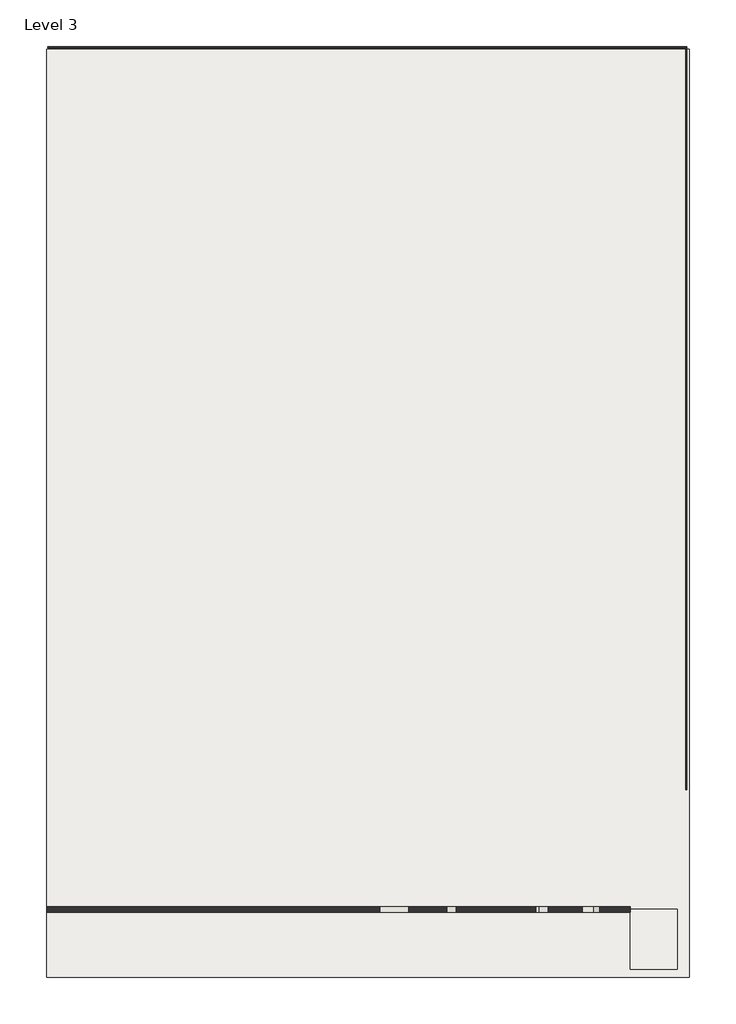
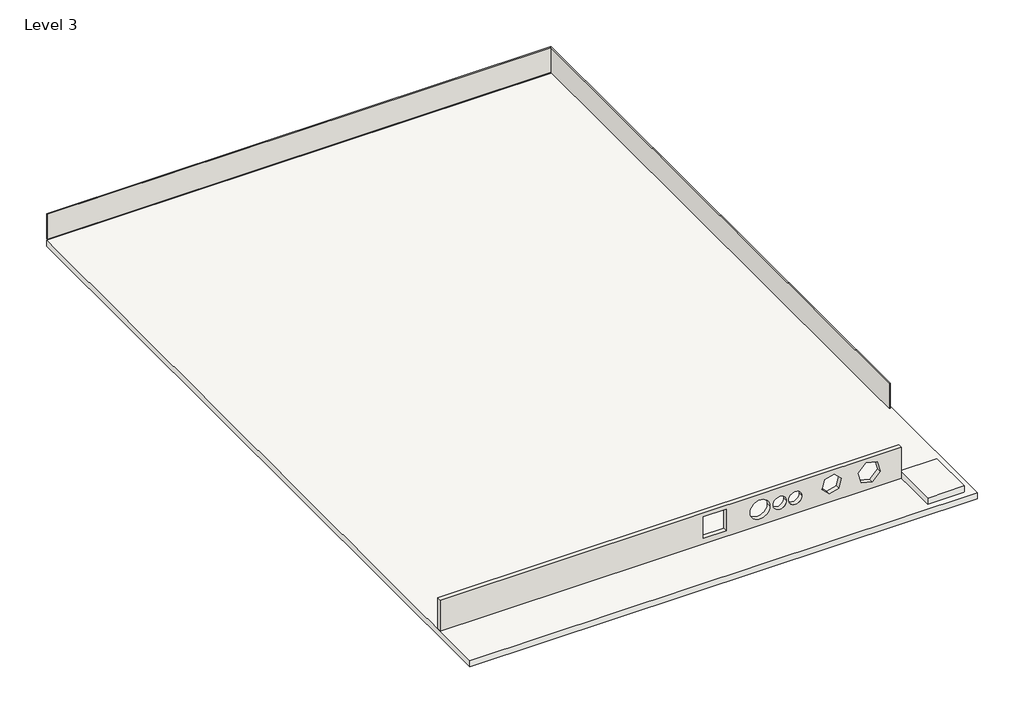
# One storey: 3 walls, 1 roof, 1 slab.
"""IFC4 building model written with IfcOpenShell, lengths in millimetres."""

from ifc_helpers import new_model, si_unit, point, frame, frame_2d, origin, place, context, project, spatial, polyline, circle_curve, trimmed, segment, composite_curve, outline, extrude, faceted_brep, element, save

model = new_model("IFC4")

# Units and contexts
model_context = context("Model", 3, world=origin())
ifc_project = project(units=[si_unit("LENGTHUNIT", "METRE", prefix="MILLI")], contexts=[model_context])

# Site, building, storey
site = spatial("IfcSite", under=ifc_project)
building = spatial("IfcBuilding", under=site)
storey = spatial("IfcBuildingStorey", under=building, Name="Level 3", Elevation=6400.8)

# Roof
placement = place(None, origin())
element("IfcRoof", 1, ObjectType="Generic - 12\"", at=placement, inside=storey, context=model_context, shape_type="SweptSolid", body=[
    extrude(outline(polyline([(2826.3321681, -15369.7898918), (4528.1321681, -15369.7898918), (4528.1321681, -17560.5647765), (2826.3321681, -17560.5647765), (2826.3321681, -15369.7898918)])), frame((0.0, 0.0, 6400.8), z_axis=(0.0, 0.0, 1.0), x_axis=(1.0, 0.0, 0.0)), (0.0, 0.0, 1.0), 304.8),
])

# Slab
element("IfcSlab", 2, ObjectType="Generic - 12\"", at=placement, inside=storey, context=model_context, shape_type="SweptSolid", body=[
    extrude(outline(polyline([(4966.8049896, 16050.0101082), (4966.8049896, -17852.8166755), (-18502.7950104, -17852.8166755), (-18502.7950104, 16050.0101082), (4966.8049896, 16050.0101082)])), frame((0.0, 0.0, 6096.0), z_axis=(0.0, 0.0, 1.0), x_axis=(1.0, 0.0, 0.0)), (0.0, 0.0, 1.0), 304.8),
])

# Walls
element("IfcWall", 3, at=placement, inside=storey, context=model_context, shape_type="Brep", body=[
    faceted_brep([(4890.6049896, -11000.9898918, 6400.8), (4890.6049896, 16151.6101082, 6400.8), (4890.6049896, 16151.6101082, 7620.0), (4890.6049896, -11000.9898918, 7620.0), (4839.8049896, -11000.9898918, 6400.8), (4839.8049896, -11000.9898918, 7620.0), (4839.8049896, 16100.8101082, 7620.0), (4839.8049896, 16151.6101082, 7620.0), (4839.8049896, 16151.6101082, 6400.8), (4839.8049896, 16100.8101082, 6400.8)], [[[0, 1, 2, 3]], [[4, 5, 6, 7, 8, 9]], [[1, 0, 4, 9, 8]], [[3, 2, 7, 6, 5]], [[0, 3, 5, 4]], [[2, 1, 8, 7]]]),
])
element("IfcWall", 4, at=placement, inside=storey, context=model_context, shape_type="SweptSolid", body=[
    extrude(outline(polyline([(-18451.9950104, 16151.6101082), (4839.8049896, 16151.6101082), (4839.8049896, 16100.8101082), (-18451.9950104, 16100.8101082), (-18451.9950104, 16151.6101082)])), frame((0.0, 0.0, 6400.8), z_axis=(0.0, 0.0, 1.0), x_axis=(1.0, 0.0, 0.0)), (0.0, 0.0, 1.0), 1219.2),
])
element("IfcWall", 5, ObjectType="Generic - 8\"", at=placement, inside=storey, context=model_context, shape_type="SweptSolid", body=[
    extrude(outline(polyline([(6400.8, 2826.3321681), (7924.8, 2826.3321681), (7924.8, -18502.7950104), (6400.8, -18502.7950104), (6400.8, 2826.3321681)]), holes=[polyline([(7740.3253268, -5264.4087327), (6673.5253268, -5264.4087327), (6673.5253268, -6331.2087327), (7740.3253268, -6331.2087327), (7740.3253268, -5264.4087327)]), composite_curve([segment(trimmed(circle_curve(frame_2d((7179.1990687, -3713.8387118)), 457.2), [point((7179.1990687, -4171.0387118))], [point((7179.1990687, -3256.6387118))], True, "CARTESIAN"), True, "CONTINUOUS"), segment(trimmed(circle_curve(frame_2d((7179.1990687, -3713.8387118)), 457.2), [point((7179.1990687, -3256.6387118))], [point((7179.1990687, -4171.0387118))], True, "CARTESIAN"), True, "CONTINUOUS")], self_intersect=False), composite_curve([segment(trimmed(circle_curve(frame_2d((7179.1990687, -2799.4387118)), 304.8), [point((7179.1990687, -3104.2387118))], [point((7179.1990687, -2494.6387118))], True, "CARTESIAN"), True, "CONTINUOUS"), segment(trimmed(circle_curve(frame_2d((7179.1990687, -2799.4387118)), 304.8), [point((7179.1990687, -2494.6387118))], [point((7179.1990687, -3104.2387118))], True, "CARTESIAN"), True, "CONTINUOUS")], self_intersect=False), composite_curve([segment(trimmed(circle_curve(frame_2d((7166.4122392, -2081.2144905)), 304.8), [point((7166.4122392, -2386.0144905))], [point((7166.4122392, -1776.4144905))], True, "CARTESIAN"), True, "CONTINUOUS"), segment(trimmed(circle_curve(frame_2d((7166.4122392, -2081.2144905)), 304.8), [point((7166.4122392, -1776.4144905))], [point((7166.4122392, -2386.0144905))], True, "CARTESIAN"), True, "CONTINUOUS")], self_intersect=False), polyline([(7375.9960597, 52.1524453), (6934.374772, -66.1796221), (6816.0427045, -507.8009099), (7139.3319249, -831.0901303), (7580.9532127, -712.7580628), (7699.2852801, -271.1367751), (7375.9960597, 52.1524453)]), polyline([(7599.8956744, 1709.9898409), (7089.9553356, 1846.6279429), (6716.6530988, 1473.3257061), (6853.2912008, 963.3853673), (7363.2315396, 826.7472654), (7736.5337764, 1200.0495022), (7599.8956744, 1709.9898409)])]), frame((0.0, -15471.3898918, 0.0), z_axis=(0.0, 1.0, 0.0), x_axis=(0.0, 0.0, 1.0)), (0.0, 0.0, 1.0), 203.2),
])

save(model, "model.ifc")

# Revit data of these elements
# Type "Generic - 12\""
#   Assembly Code = "B1020"
#   Layers, outside or top first: 1' - 0" no material (function 1)
# Type "Generic - 12\""
#   Assembly Code = "B1010"
#   Function = 0
#   Layers, outside or top first: 1' - 0" no material (function 1)
# Type
#   Assembly Code = "B2010"
#   Layers, outside or top first: 0' - 1 1/2" "Softwood, Lumber" (function 1); 0' - 0 1/2" "Door - Frame" (function 5)
# Type "Generic - 8\""
#   Assembly Code = "B2010"
#   Layers, outside or top first: 0' - 8" no material (function 1)
# Element 1 (IfcRoof, "Generic - 12\"")
#   built-in parameter 1001705 = 22 (stored number, unit not read)
#   built-in parameter 1001710 = 33615
#   Phase Created = New Construction
#   Materials on its faces: "Default Roof"
# Element 2 (IfcSlab, "Generic - 12\"")
#   Height Offset From Level = 0' - 0"
#   Phase Created = New Construction
#   Materials on its faces: "Default Floor"
# Elements 3, 4 (IfcWall)
#   Top Offset = 0' - 0"
#   Base Offset = 0' - 0"
#   Unconnected Height = 4' - 0"
#   wall height = 4' - 0"
#   Phase Created = New Construction
#   Base Constraint = Level 3
#   Materials on its faces: "Default Wall", "Door - Frame", "Softwood, Lumber"
# Element 5 (IfcWall, "Generic - 8\"")
#   Top Offset = 0' - 0"
#   Base Offset = 0' - 0"
#   Unconnected Height = 5' - 0"
#   wall height = 5' - 0"
#   Phase Created = New Construction
#   Base Constraint = Level 3
#   Materials on its faces: "Default Wall"
# Materials
#   "Softwood, Lumber": class "Wood", colour RGB 223 192 134, transparency 0, Description = "Pinus Echinata", Cost = 0
#   "Door - Frame": colour RGB 118 70 51, transparency 0
#   "Default Roof": colour RGB 88 101 114, transparency 0
#   "Default Floor": colour RGB 128 128 128, transparency 0
#   "Default Wall": colour RGB 128 128 128, transparency 0
